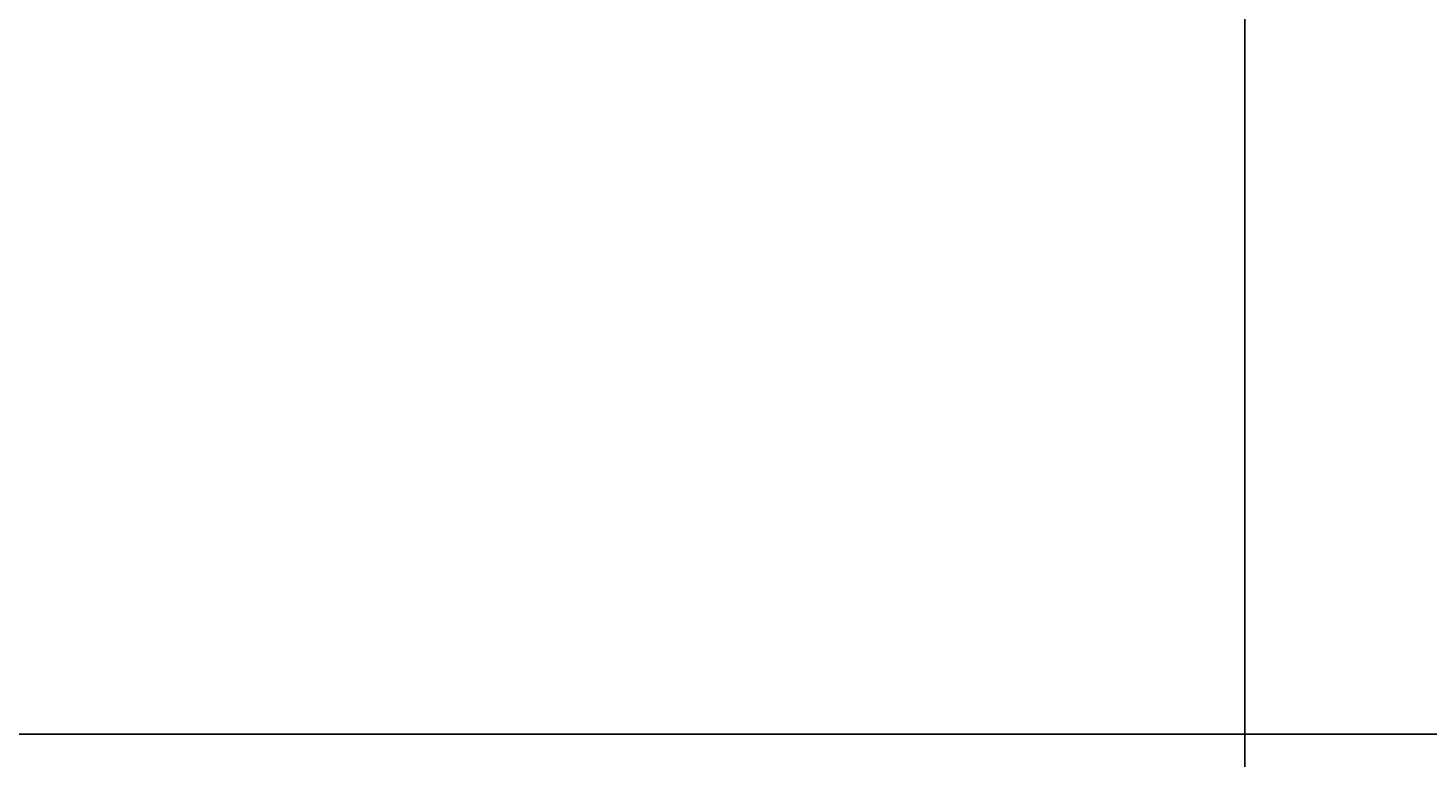
# Model space of a CAD drawing. Units: inches. Extents: x -301 to 715, y -607 to 364.
# Tile 11 of 141: x -19 to 18, y -512 to -493. Entities that reach past the tile are written whole.
import ezdxf

# ---------------------------------------------------------------- set-up
doc = ezdxf.new("R2010")
doc.units = ezdxf.units.IN
doc.header["$MEASUREMENT"] = 0
doc.layers.add('A-ANNO-DIMS', color=2, linetype='Continuous', lineweight=18)
doc.styles.get("Standard").update_dxf_attribs({"font": 'arial.ttf'})
doc.dimstyles.get("Standard").update_dxf_attribs({"dimtxt": 0.18, "dimasz": 0.18, "dimexe": 0.18, "dimexo": 0.0625, "dimgap": 0.09, "dimtad": 0, "dimtih": 1, "dimtoh": 1, "dimdec": 1, "dimzin": 0, "dimdsep": 46, "dimlunit": 4, "dimtxsty": 'Standard', "dimcen": 0.09, "dimclrd": 3, "dimclre": 4, "dimclrt": 6, "dimadec": 0, "dimazin": 0, "dimtfac": 1, "dimtdec": 1, "dimtofl": 0, "dimtmove": 0, "dimatfit": 3, "dimfxl": 1, "dimtfill": 2, "dimtfillclr": 51, "dimtolj": 1, "dimtzin": 0, "dimarcsym": 0})

# ---------------------------------------------------------------- blocks, each defined once
blk = doc.blocks.new('*D176')
at = {"layer": 'A-ANNO-DIMS', "color": 4, "lineweight": -2, "transparency": 16777216}
for p, q in [((148.28, -324.477), (215.605, -324.477)), ((-15.22, -540.477), (215.605, -540.477))]:
    blk.add_line(p, q, dxfattribs=at)
at = {"layer": 'A-ANNO-DIMS', "color": 3, "lineweight": -2, "transparency": 16777216}
for p, q in [((215.425, -324.657), (215.425, -432.296)), ((215.425, -540.297), (215.425, -432.659))]:
    blk.add_line(p, q, dxfattribs=at)
at = {"layer": 'A-ANNO-DIMS', "color": 3, "transparency": 16777216}
for points in [[(215.395, -324.657), (215.455, -324.657), (215.425, -324.477)], [(215.395, -540.297), (215.455, -540.297), (215.425, -540.477)]]:
    blk.add_solid(points, dxfattribs=at)
at = {"layer": 'Defpoints', "color": 0, "transparency": 16777216}
for p in [(148.218, -324.477), (-15.282, -540.477), (215.425, -540.477)]:
    blk.add_point(p, dxfattribs=at)
at = {"layer": 'A-ANNO-DIMS', "color": 6, "transparency": 16777216, "insert": (215.425, -432.477), "char_height": 0.18, "attachment_point": 5, "bg_fill": 1, "box_fill_scale": 1.25, "bg_fill_color": 51, "bg_fill_transparency": 0}
blk.add_mtext('\\A1;18\'-0"', dxfattribs=at)
blk = doc.blocks.new('*D180')
at = {"layer": 'A-ANNO-DIMS', "color": 4, "lineweight": -2, "transparency": 16777216}
for p, q in [((-35.282, -463.54), (-35.282, -573.809)), ((12.718, -463.54), (12.718, -573.809))]:
    blk.add_line(p, q, dxfattribs=at)
at = {"layer": 'A-ANNO-DIMS', "color": 3, "lineweight": -2, "transparency": 16777216}
for p, q in [((-35.102, -573.629), (-11.615, -573.629)), ((12.538, -573.629), (-10.949, -573.629))]:
    blk.add_line(p, q, dxfattribs=at)
at = {"layer": 'A-ANNO-DIMS', "color": 3, "transparency": 16777216}
for points in [[(-35.102, -573.599), (-35.102, -573.659), (-35.282, -573.629)], [(12.538, -573.599), (12.538, -573.659), (12.718, -573.629)]]:
    blk.add_solid(points, dxfattribs=at)
at = {"layer": 'Defpoints', "color": 0, "transparency": 16777216}
for p in [(-35.282, -463.477), (12.718, -463.477), (12.718, -573.629)]:
    blk.add_point(p, dxfattribs=at)
at = {"layer": 'A-ANNO-DIMS', "color": 6, "transparency": 16777216, "insert": (-11.282, -573.629), "char_height": 0.18, "attachment_point": 5, "bg_fill": 1, "box_fill_scale": 1.25, "bg_fill_color": 51, "bg_fill_transparency": 0}
blk.add_mtext('\\A1;4\'-0"', dxfattribs=at)
blk = doc.blocks.new('*D181')
at = {"layer": 'A-ANNO-DIMS', "color": 4, "lineweight": -2, "transparency": 16777216}
for p, q in [((48.468, -433.54), (48.468, -573.809)), ((12.718, -463.54), (12.718, -573.809))]:
    blk.add_line(p, q, dxfattribs=at)
at = {"layer": 'A-ANNO-DIMS', "color": 3, "lineweight": -2, "transparency": 16777216}
for p, q in [((12.898, -573.629), (30.264, -573.629)), ((48.288, -573.629), (30.922, -573.629))]:
    blk.add_line(p, q, dxfattribs=at)
at = {"layer": 'A-ANNO-DIMS', "color": 3, "transparency": 16777216}
for points in [[(12.898, -573.599), (12.898, -573.659), (12.718, -573.629)], [(48.288, -573.599), (48.288, -573.659), (48.468, -573.629)]]:
    blk.add_solid(points, dxfattribs=at)
at = {"layer": 'Defpoints', "color": 0, "transparency": 16777216}
for p in [(48.468, -433.477), (12.718, -463.477), (48.468, -573.629)]:
    blk.add_point(p, dxfattribs=at)
at = {"layer": 'A-ANNO-DIMS', "color": 6, "transparency": 16777216, "insert": (30.593, -573.629), "char_height": 0.18, "attachment_point": 5, "bg_fill": 1, "box_fill_scale": 1.25, "bg_fill_color": 51, "bg_fill_transparency": 0}
blk.add_mtext('\\A1;3\'-0"', dxfattribs=at)
blk = doc.blocks.new('*D190')
at = {"layer": 'A-ANNO-DIMS', "color": 4, "lineweight": -2, "transparency": 16777216}
for p, q in [((129.193, -481.477), (-266.112, -481.477)), ((124.193, -511.477), (-266.112, -511.477))]:
    blk.add_line(p, q, dxfattribs=at)
at = {"layer": 'A-ANNO-DIMS', "color": 3, "lineweight": -2, "transparency": 16777216}
for p, q in [((-265.932, -481.657), (-265.932, -496.296)), ((-265.932, -511.297), (-265.932, -496.659))]:
    blk.add_line(p, q, dxfattribs=at)
at = {"layer": 'A-ANNO-DIMS', "color": 3, "transparency": 16777216}
for points in [[(-265.962, -481.657), (-265.902, -481.657), (-265.932, -481.477)], [(-265.962, -511.297), (-265.902, -511.297), (-265.932, -511.477)]]:
    blk.add_solid(points, dxfattribs=at)
at = {"layer": 'Defpoints', "color": 0, "transparency": 16777216}
for p in [(129.255, -481.477), (-265.932, -511.477), (124.255, -511.477)]:
    blk.add_point(p, dxfattribs=at)
at = {"layer": 'A-ANNO-DIMS', "color": 6, "transparency": 16777216, "insert": (-265.932, -496.477), "char_height": 0.18, "attachment_point": 5, "bg_fill": 1, "box_fill_scale": 1.25, "bg_fill_color": 51, "bg_fill_transparency": 0}
blk.add_mtext('\\A1;2\'-6"', dxfattribs=at)
blk = doc.blocks.new('*D191')
at = {"layer": 'A-ANNO-DIMS', "color": 4, "lineweight": -2, "transparency": 16777216}
for p, q in [((129.193, -481.477), (-266.112, -481.477)), ((114.193, -540.477), (-266.112, -540.477))]:
    blk.add_line(p, q, dxfattribs=at)
at = {"layer": 'A-ANNO-DIMS', "color": 3, "lineweight": -2, "transparency": 16777216}
for p, q in [((-265.932, -481.657), (-265.932, -510.797)), ((-265.932, -540.297), (-265.932, -511.158))]:
    blk.add_line(p, q, dxfattribs=at)
at = {"layer": 'A-ANNO-DIMS', "color": 3, "transparency": 16777216}
for points in [[(-265.962, -481.657), (-265.902, -481.657), (-265.932, -481.477)], [(-265.962, -540.297), (-265.902, -540.297), (-265.932, -540.477)]]:
    blk.add_solid(points, dxfattribs=at)
at = {"layer": 'Defpoints', "color": 0, "transparency": 16777216}
for p in [(129.255, -481.477), (-265.932, -540.477), (114.255, -540.477)]:
    blk.add_point(p, dxfattribs=at)
at = {"layer": 'A-ANNO-DIMS', "color": 6, "transparency": 16777216, "insert": (-265.932, -510.977), "char_height": 0.18, "attachment_point": 5, "bg_fill": 1, "box_fill_scale": 1.25, "bg_fill_color": 51, "bg_fill_transparency": 0}
blk.add_mtext('\\A1;4\'-11"', dxfattribs=at)

msp = doc.modelspace()

# ---------------------------------------------------------------- dimensions: what is measured, and where the dimension line sits
at = {"layer": 'A-ANNO-DIMS'}
for base, p1, p2, picture, middle in [((215.425, -540.477), (148.218, -324.477), (-15.282, -540.477), '*D176', (215.425, -432.477)), ((-265.932, -540.477), (129.255, -481.477), (114.255, -540.477), '*D191', (-265.932, -510.977)), ((-265.932, -511.477), (129.255, -481.477), (124.255, -511.477), '*D190', (-265.932, -496.477))]:
    dim = msp.add_linear_dim(base=base, p1=p1, p2=p2, angle=90, dimstyle='Standard', override={"dimdec": 1, "dimlfac": 1, "dimrnd": 0, "dimzin": 1, "dimdsep": 46, "dimlunit": 4, "dimfrac": 2}, dxfattribs=at)
    dim.commit()
    dim.dimension.update_dxf_attribs({"geometry": picture, "text_midpoint": middle})
for base, p1, p2, picture, middle in [((48.467984, -573.628877), (12.717984, -463.47741), (48.467984, -433.47741), '*D181', (30.592984, -573.628877)), ((12.718, -573.629), (-35.282, -463.477), (12.718, -463.477), '*D180', (-11.282, -573.629))]:
    dim = msp.add_linear_dim(base=base, p1=p1, p2=p2, dimstyle='Standard', override={"dimdec": 1, "dimlfac": 1, "dimrnd": 0, "dimzin": 1, "dimdsep": 46, "dimlunit": 4, "dimfrac": 2}, dxfattribs=at)
    dim.commit()
    dim.dimension.update_dxf_attribs({"geometry": picture, "text_midpoint": middle})

doc.saveas('drawing.dxf')
